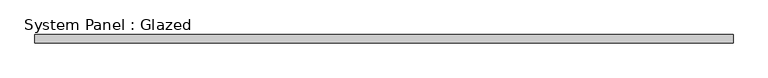
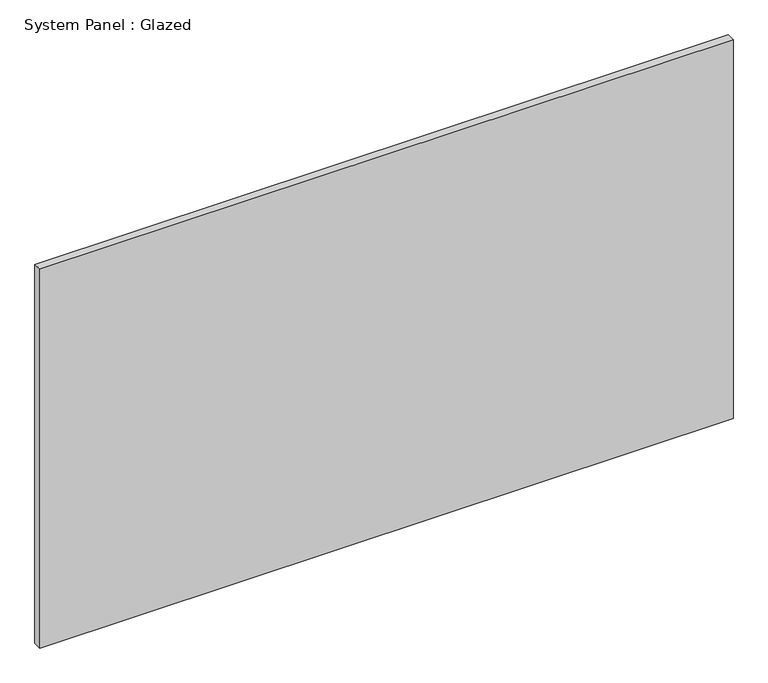
"""IFC4 building model written with IfcOpenShell, lengths in millimetres: plate geometry, System Panel : Glazed."""

from ifc_helpers import new_model, si_unit, origin, origin_with_axes, place, context, project, spatial, polyline, outline, extrude, source, transform, mapped, element, save


def system_panel_glazed_5b5c8ea9(model_context):
    return source(origin(), model_context, "Body", "SweptSolid", [
        extrude(outline(polyline([(1054.1, 19.05), (-1054.1, 19.05), (-1054.1, 44.45), (1054.1, 44.45), (1054.1, 19.05)])), origin_with_axes(), (0.0, 0.0, 1.0), 1219.2),
    ])


if __name__ == "__main__":
    model = new_model("IFC4")
    model_context = context("Model", 3, world=origin())
    ifc_project = project(units=[si_unit("LENGTHUNIT", "METRE", prefix="MILLI")], contexts=[model_context])
    site = spatial("IfcSite", under=ifc_project)
    building = spatial("IfcBuilding", under=site)
    placement = place(None, origin())
    system_panel_glazed_shape = system_panel_glazed_5b5c8ea9(model_context)
    element("IfcPlate", 1, ObjectType="System Panel : Glazed", at=placement, inside=building, context=model_context, shape_type="MappedRepresentation", body=[
        mapped(system_panel_glazed_shape, transform((0.0, 0.0, 0.0), x_axis=(1.0, 0.0, 0.0), y_axis=(0.0, 1.0, 0.0), z_axis=(0.0, 0.0, 1.0))),
    ])
    save(model, "model.ifc")

# Revit data of these elements
# Type "System Panel : Glazed"
#   Construction Type Id = "GSP4R"
#   Analytic Construction = "1/8 in Pilkington single glazing"
#   Visual Light Transmittance = 0.9
#   Solar Heat Gain Coefficient = 0.86
#   Heat Transfer Coefficient (U) = 1.18115 BTU/(h·ft²·°F)
# Element 1 (IfcPlate, "System Panel : Glazed")
#   Materials on its faces: "Glass"
# Materials
#   "Glass": class "Glass", colour RGB 0 128 192, transparency 0.75, Description = "Soda Lime Glass", Cost = 0
